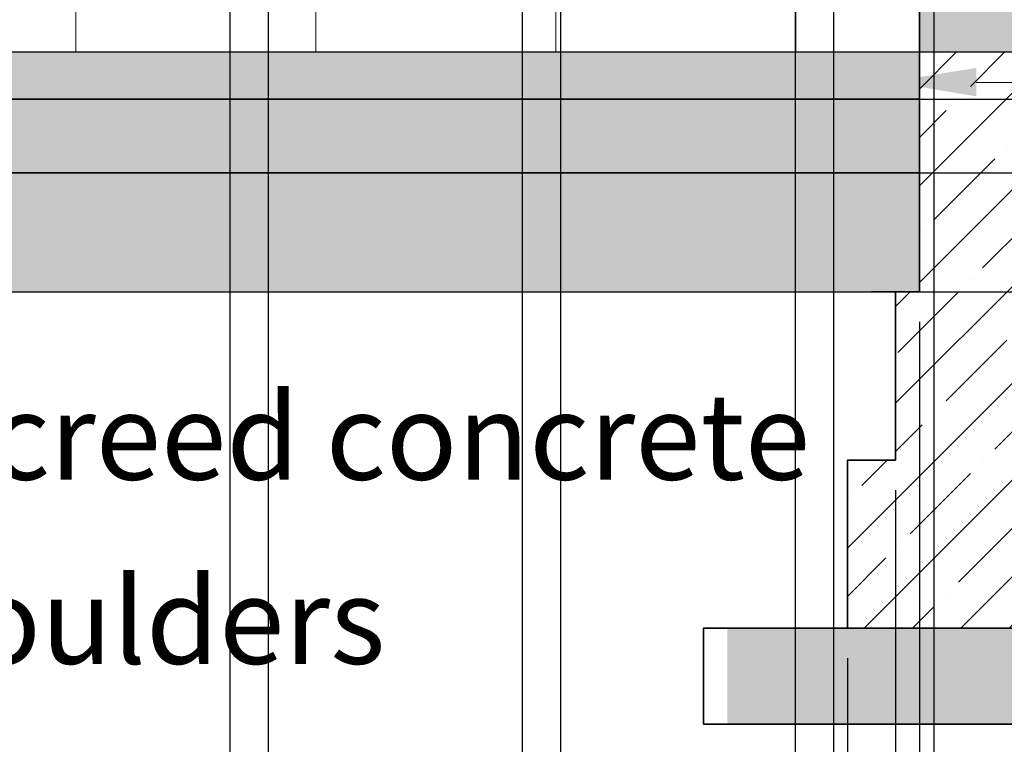
# Model space of a CAD drawing. Units: metres. Extents: x 22.1 to 34.4, y 4.4 to 12.4.
# Tile 4 of 8: x 29.6 to 31.7, y 7 to 8.5. Entities that reach past the tile are written whole.
import ezdxf
from ezdxf import colors
from ezdxf.entities.mleader import LeaderData, LeaderLine
from ezdxf.math import Vec2, Vec3

# ---------------------------------------------------------------- set-up
doc = ezdxf.new("R2010")
doc.units = ezdxf.units.M
doc.header["$MEASUREMENT"] = 0
for name, color, linetype, lineweight in [('A-ANNO-DIMS', 2, 'Continuous', 18), ('A-ANNO-TEXT', 7, 'Continuous', 18), ('A-FLOR', 3, 'Continuous', 25), ('A-FLOR-PATT', 252, 'Continuous', 13), ('S-FNDN', 1, 'Continuous', 35), ('S-FNDN-PATT', 8, 'Continuous', 13), ('S-SLAB-PATT', 8, 'Continuous', 13)]:
    doc.layers.add(name, color=color, linetype=linetype, lineweight=lineweight)
doc.styles.get("Standard").update_dxf_attribs({"font": 'arial.ttf'})
doc.dimstyles.get("Standard").update_dxf_attribs({"dimtxt": 0.18, "dimasz": 0.18, "dimexe": 0.18, "dimexo": 0.0625, "dimgap": 0.09, "dimtad": 0, "dimtih": 1, "dimtoh": 1, "dimzin": 0, "dimdsep": 46, "dimtxsty": 'Standard', "dimcen": 0.09, "dimadec": 0, "dimazin": 0, "dimtfac": 1, "dimtofl": 0, "dimtmove": 0, "dimatfit": 3, "dimfxl": 1, "dimtolj": 1, "dimtzin": 0, "dimarcsym": 0})

# ---------------------------------------------------------------- blocks, each defined once
blk = doc.blocks.new('*D7')
at = {"layer": 'A-ANNO-DIMS', "color": 0, "lineweight": -2, "transparency": 16777216}
for p, q in [((31.0581, 6.9474), (31.0581, 5.2806)), ((32.2581, 6.9474), (32.2581, 5.2806)), ((31.0581, 5.4606), (30.8781, 5.4606)), ((32.0781, 5.4606), (31.2381, 5.4606))]:
    blk.add_line(p, q, dxfattribs=at)
at = {"layer": 'A-ANNO-DIMS', "color": 0, "transparency": 16777216}
for points in [[(31.2381, 5.4906), (31.2381, 5.4306), (31.0581, 5.4606)], [(32.0781, 5.4906), (32.0781, 5.4306), (32.2581, 5.4606)]]:
    blk.add_solid(points, dxfattribs=at)
at = {"layer": 'Defpoints', "color": 0, "transparency": 16777216}
for p in [(31.0581, 7.0099), (32.2581, 7.0099), (32.2581, 5.4606)]:
    blk.add_point(p, dxfattribs=at)
at = {"layer": 'A-ANNO-DIMS', "color": 0, "transparency": 16777216, "insert": (30.5631, 5.4606), "char_height": 0.18, "attachment_point": 5}
blk.add_mtext('\\A1;1.20', dxfattribs=at)
blk = doc.blocks.new('*D8')
at = {"layer": 'A-ANNO-DIMS', "color": 0, "lineweight": -2, "transparency": 16777216}
for p, q in [((31.3581, 7.1474), (31.3581, 5.6208)), ((31.9581, 7.1474), (31.9581, 5.6208)), ((31.3581, 5.8008), (30.8904, 5.8008)), ((31.7781, 5.8008), (31.5381, 5.8008))]:
    blk.add_line(p, q, dxfattribs=at)
at = {"layer": 'A-ANNO-DIMS', "color": 0, "transparency": 16777216}
for points in [[(31.5381, 5.8308), (31.5381, 5.7708), (31.3581, 5.8008)], [(31.7781, 5.8308), (31.7781, 5.7708), (31.9581, 5.8008)]]:
    blk.add_solid(points, dxfattribs=at)
at = {"layer": 'Defpoints', "color": 0, "transparency": 16777216}
for p in [(31.3581, 7.2099), (31.9581, 7.2099), (31.9581, 5.8008)]:
    blk.add_point(p, dxfattribs=at)
at = {"layer": 'A-ANNO-DIMS', "color": 0, "transparency": 16777216, "insert": (30.5669, 5.8008), "char_height": 0.18, "attachment_point": 5}
blk.add_mtext('\\A1;0.60', dxfattribs=at)
blk = doc.blocks.new('*D9')
at = {"layer": 'A-ANNO-DIMS', "color": 0, "lineweight": -2, "transparency": 16777216}
for p, q in [((31.4581, 7.4974), (31.4581, 5.952)), ((31.8581, 7.4974), (31.8581, 5.952)), ((31.2781, 6.132), (30.8756, 6.132)), ((32.0381, 6.132), (32.2181, 6.132))]:
    blk.add_line(p, q, dxfattribs=at)
at = {"layer": 'A-ANNO-DIMS', "color": 0, "transparency": 16777216}
for points in [[(31.2781, 6.162), (31.2781, 6.102), (31.4581, 6.132)], [(32.0381, 6.162), (32.0381, 6.102), (31.8581, 6.132)]]:
    blk.add_solid(points, dxfattribs=at)
at = {"layer": 'Defpoints', "color": 0, "transparency": 16777216}
for p in [(31.4581, 7.5599), (31.8581, 7.5599), (31.8581, 6.132)]:
    blk.add_point(p, dxfattribs=at)
at = {"layer": 'A-ANNO-DIMS', "color": 0, "transparency": 16777216, "insert": (30.5521, 6.132), "char_height": 0.18, "attachment_point": 5}
blk.add_mtext('\\A1;0.40', dxfattribs=at)
blk = doc.blocks.new('*D10')
at = {"layer": 'A-ANNO-DIMS', "color": 0, "lineweight": -2, "transparency": 16777216}
for p, q in [((31.5081, 7.8474), (31.5081, 6.2035)), ((31.8081, 7.8474), (31.8081, 6.2035)), ((31.3281, 6.3835), (30.8854, 6.3835)), ((31.9881, 6.3835), (32.1681, 6.3835))]:
    blk.add_line(p, q, dxfattribs=at)
at = {"layer": 'A-ANNO-DIMS', "color": 0, "transparency": 16777216}
for points in [[(31.3281, 6.4135), (31.3281, 6.3535), (31.5081, 6.3835)], [(31.9881, 6.4135), (31.9881, 6.3535), (31.8081, 6.3835)]]:
    blk.add_solid(points, dxfattribs=at)
at = {"layer": 'Defpoints', "color": 0, "transparency": 16777216}
for p in [(31.5081, 7.9099), (31.8081, 7.9099), (31.8081, 6.3835)]:
    blk.add_point(p, dxfattribs=at)
at = {"layer": 'A-ANNO-DIMS', "color": 0, "transparency": 16777216, "insert": (30.562, 6.3835), "char_height": 0.18, "attachment_point": 5}
blk.add_mtext('\\A1;0.30', dxfattribs=at)
blk = doc.blocks.new('*D23')
at = {"layer": 'A-ANNO-DIMS', "color": 0, "lineweight": -2, "transparency": 16777216}
for p, q in [((28.0901, 11.4474), (28.0901, 6.2449)), ((31.5381, 11.4474), (31.5381, 6.2449)), ((28.2701, 6.4249), (29.4202, 6.4249)), ((31.3581, 6.4249), (30.2079, 6.4249))]:
    blk.add_line(p, q, dxfattribs=at)
at = {"layer": 'A-ANNO-DIMS', "color": 0, "transparency": 16777216}
for points in [[(28.2701, 6.4549), (28.2701, 6.3949), (28.0901, 6.4249)], [(31.3581, 6.4549), (31.3581, 6.3949), (31.5381, 6.4249)]]:
    blk.add_solid(points, dxfattribs=at)
at = {"layer": 'Defpoints', "color": 0, "transparency": 16777216}
for p in [(28.0901, 11.5099), (31.5381, 11.5099), (31.5381, 6.4249)]:
    blk.add_point(p, dxfattribs=at)
at = {"layer": 'A-ANNO-DIMS', "color": 0, "transparency": 16777216, "insert": (29.8141, 6.4249), "char_height": 0.18, "attachment_point": 5}
blk.add_mtext('\\A1;3.448', dxfattribs=at)
blk = doc.blocks.new('*D27')
at = {"layer": 'A-ANNO-DIMS', "color": 0, "lineweight": -2, "transparency": 16777216}
for p, q in [((31.5381, 11.4474), (31.5381, 6.2449)), ((31.7781, 11.4474), (31.7781, 6.2449)), ((31.3581, 6.4249), (31.1781, 6.4249)), ((31.9581, 6.4249), (32.1381, 6.4249))]:
    blk.add_line(p, q, dxfattribs=at)
at = {"layer": 'A-ANNO-DIMS', "color": 0, "transparency": 16777216}
for points in [[(31.3581, 6.4549), (31.3581, 6.3949), (31.5381, 6.4249)], [(31.9581, 6.4549), (31.9581, 6.3949), (31.7781, 6.4249)]]:
    blk.add_solid(points, dxfattribs=at)
at = {"layer": 'Defpoints', "color": 0, "transparency": 16777216}
for p in [(31.5381, 11.5099), (31.7781, 11.5099), (31.7781, 6.4249)]:
    blk.add_point(p, dxfattribs=at)
at = {"layer": 'A-ANNO-DIMS', "color": 0, "transparency": 16777216, "insert": (32.4615, 6.4249), "char_height": 0.18, "attachment_point": 5}
blk.add_mtext('\\A1;0.24', dxfattribs=at)
blk = doc.blocks.new('*D28')
at = {"layer": 'A-ANNO-DIMS', "color": 0, "lineweight": -2, "transparency": 16777216}
for p, q in [((31.7781, 11.4474), (31.7781, 6.2449)), ((31.9781, 11.4474), (31.9781, 6.2449)), ((31.5981, 6.4249), (31.4181, 6.4249)), ((32.1581, 6.4249), (32.3381, 6.4249))]:
    blk.add_line(p, q, dxfattribs=at)
at = {"layer": 'A-ANNO-DIMS', "color": 0, "transparency": 16777216}
for points in [[(31.5981, 6.4549), (31.5981, 6.3949), (31.7781, 6.4249)], [(32.1581, 6.4549), (32.1581, 6.3949), (31.9781, 6.4249)]]:
    blk.add_solid(points, dxfattribs=at)
at = {"layer": 'Defpoints', "color": 0, "transparency": 16777216}
for p in [(31.7781, 11.5099), (31.9781, 11.5099), (31.9781, 6.4249)]:
    blk.add_point(p, dxfattribs=at)
at = {"layer": 'A-ANNO-DIMS', "color": 0, "transparency": 16777216, "insert": (32.6615, 6.4249), "char_height": 0.18, "attachment_point": 5}
blk.add_mtext('\\A1;0.20', dxfattribs=at)
blk = doc.blocks.new('*D33')
at = {"layer": 'A-ANNO-DIMS', "color": 0, "lineweight": -2, "transparency": 16777216}
for p, q in [((31.5381, 11.4474), (31.5381, 6.2449)), ((31.3293, 10.5774), (31.3293, 6.2449)), ((31.1493, 6.4249), (30.9693, 6.4249)), ((31.7181, 6.4249), (31.8981, 6.4249))]:
    blk.add_line(p, q, dxfattribs=at)
at = {"layer": 'A-ANNO-DIMS', "color": 0, "transparency": 16777216}
for points in [[(31.1493, 6.4549), (31.1493, 6.3949), (31.3293, 6.4249)], [(31.7181, 6.4549), (31.7181, 6.3949), (31.5381, 6.4249)]]:
    blk.add_solid(points, dxfattribs=at)
at = {"layer": 'Defpoints', "color": 0, "transparency": 16777216}
for p in [(31.5381, 11.5099), (31.3293, 10.6399), (31.5381, 6.4249)]:
    blk.add_point(p, dxfattribs=at)
at = {"layer": 'A-ANNO-DIMS', "color": 0, "transparency": 16777216, "insert": (32.2045, 6.4249), "char_height": 0.18, "attachment_point": 5}
blk.add_mtext('\\A1;0.21', dxfattribs=at)
blk = doc.blocks.new('*D34')
at = {"layer": 'A-ANNO-DIMS', "color": 0, "lineweight": -2, "transparency": 16777216}
for p, q in [((28.8933, 9.3614), (28.8933, 6.2449)), ((31.3293, 9.3614), (31.3293, 6.2449)), ((29.0733, 6.4249), (29.7162, 6.4249)), ((31.1493, 6.4249), (30.5065, 6.4249))]:
    blk.add_line(p, q, dxfattribs=at)
at = {"layer": 'A-ANNO-DIMS', "color": 0, "transparency": 16777216}
for points in [[(29.0733, 6.4549), (29.0733, 6.3949), (28.8933, 6.4249)], [(31.1493, 6.4549), (31.1493, 6.3949), (31.3293, 6.4249)]]:
    blk.add_solid(points, dxfattribs=at)
at = {"layer": 'Defpoints', "color": 0, "transparency": 16777216}
for p in [(28.8933, 9.4239), (31.3293, 9.4239), (31.3293, 6.4249)]:
    blk.add_point(p, dxfattribs=at)
at = {"layer": 'A-ANNO-DIMS', "color": 0, "transparency": 16777216, "insert": (30.1113, 6.4249), "char_height": 0.18, "attachment_point": 5}
blk.add_mtext('\\A1;2.436', dxfattribs=at)
blk = doc.blocks.new('*D35')
at = {"layer": 'A-ANNO-DIMS', "color": 0, "lineweight": -2, "transparency": 16777216}
for p, q in [((28.9733, 9.4414), (28.9733, 6.2449)), ((28.8933, 9.3614), (28.8933, 6.2449)), ((28.7133, 6.4249), (28.5333, 6.4249)), ((29.1533, 6.4249), (29.3333, 6.4249))]:
    blk.add_line(p, q, dxfattribs=at)
at = {"layer": 'A-ANNO-DIMS', "color": 0, "transparency": 16777216}
for points in [[(28.7133, 6.4549), (28.7133, 6.3949), (28.8933, 6.4249)], [(29.1533, 6.4549), (29.1533, 6.3949), (28.9733, 6.4249)]]:
    blk.add_solid(points, dxfattribs=at)
at = {"layer": 'Defpoints', "color": 0, "transparency": 16777216}
for p in [(28.9733, 9.5039), (28.8933, 9.4239), (28.9733, 6.4249)]:
    blk.add_point(p, dxfattribs=at)
at = {"layer": 'A-ANNO-DIMS', "color": 0, "transparency": 16777216, "insert": (29.6573, 6.4249), "char_height": 0.18, "attachment_point": 5}
blk.add_mtext('\\A1;0.08', dxfattribs=at)
blk = doc.blocks.new('*D36')
at = {"layer": 'A-ANNO-DIMS', "color": 0, "lineweight": -2, "transparency": 16777216}
for p, q in [((29.4623, 9.4414), (29.4623, 6.2449)), ((29.5423, 9.4414), (29.5423, 6.2449)), ((29.2823, 6.4249), (29.1023, 6.4249)), ((29.7223, 6.4249), (29.9023, 6.4249))]:
    blk.add_line(p, q, dxfattribs=at)
at = {"layer": 'A-ANNO-DIMS', "color": 0, "transparency": 16777216}
for points in [[(29.2823, 6.4549), (29.2823, 6.3949), (29.4623, 6.4249)], [(29.7223, 6.4549), (29.7223, 6.3949), (29.5423, 6.4249)]]:
    blk.add_solid(points, dxfattribs=at)
at = {"layer": 'Defpoints', "color": 0, "transparency": 16777216}
for p in [(29.4623, 9.5039), (29.5423, 9.5039), (29.5423, 6.4249)]:
    blk.add_point(p, dxfattribs=at)
at = {"layer": 'A-ANNO-DIMS', "color": 0, "transparency": 16777216, "insert": (30.2263, 6.4249), "char_height": 0.18, "attachment_point": 5}
blk.add_mtext('\\A1;0.08', dxfattribs=at)
blk = doc.blocks.new('*D37')
at = {"layer": 'A-ANNO-DIMS', "color": 0, "lineweight": -2, "transparency": 16777216}
for p, q in [((30.0713, 9.4414), (30.0713, 6.2449)), ((30.1513, 9.4414), (30.1513, 6.2449)), ((29.8913, 6.4249), (29.7113, 6.4249)), ((30.3313, 6.4249), (30.5113, 6.4249))]:
    blk.add_line(p, q, dxfattribs=at)
at = {"layer": 'A-ANNO-DIMS', "color": 0, "transparency": 16777216}
for points in [[(29.8913, 6.4549), (29.8913, 6.3949), (30.0713, 6.4249)], [(30.3313, 6.4549), (30.3313, 6.3949), (30.1513, 6.4249)]]:
    blk.add_solid(points, dxfattribs=at)
at = {"layer": 'Defpoints', "color": 0, "transparency": 16777216}
for p in [(30.0713, 9.5039), (30.1513, 9.5039), (30.1513, 6.4249)]:
    blk.add_point(p, dxfattribs=at)
at = {"layer": 'A-ANNO-DIMS', "color": 0, "transparency": 16777216, "insert": (30.8353, 6.4249), "char_height": 0.18, "attachment_point": 5}
blk.add_mtext('\\A1;0.08', dxfattribs=at)
blk = doc.blocks.new('*D38')
at = {"layer": 'A-ANNO-DIMS', "color": 0, "lineweight": -2, "transparency": 16777216}
for p, q in [((30.6803, 9.4414), (30.6803, 6.2449)), ((30.7603, 9.4414), (30.7603, 6.2449)), ((30.5003, 6.4249), (30.3203, 6.4249)), ((30.9403, 6.4249), (31.1203, 6.4249))]:
    blk.add_line(p, q, dxfattribs=at)
at = {"layer": 'A-ANNO-DIMS', "color": 0, "transparency": 16777216}
for points in [[(30.5003, 6.4549), (30.5003, 6.3949), (30.6803, 6.4249)], [(30.9403, 6.4549), (30.9403, 6.3949), (30.7603, 6.4249)]]:
    blk.add_solid(points, dxfattribs=at)
at = {"layer": 'Defpoints', "color": 0, "transparency": 16777216}
for p in [(30.6803, 9.5039), (30.7603, 9.5039), (30.7603, 6.4249)]:
    blk.add_point(p, dxfattribs=at)
at = {"layer": 'A-ANNO-DIMS', "color": 0, "transparency": 16777216, "insert": (31.4443, 6.4249), "char_height": 0.18, "attachment_point": 5}
blk.add_mtext('\\A1;0.08', dxfattribs=at)
blk = doc.blocks.new('*D39')
at = {"layer": 'A-ANNO-DIMS', "color": 0, "lineweight": -2, "transparency": 16777216}
for p, q in [((31.2493, 9.4414), (31.2493, 6.2449)), ((31.3293, 9.3614), (31.3293, 6.2449)), ((31.0693, 6.4249), (30.8893, 6.4249)), ((31.5093, 6.4249), (31.6893, 6.4249))]:
    blk.add_line(p, q, dxfattribs=at)
at = {"layer": 'A-ANNO-DIMS', "color": 0, "transparency": 16777216}
for points in [[(31.0693, 6.4549), (31.0693, 6.3949), (31.2493, 6.4249)], [(31.5093, 6.4549), (31.5093, 6.3949), (31.3293, 6.4249)]]:
    blk.add_solid(points, dxfattribs=at)
at = {"layer": 'Defpoints', "color": 0, "transparency": 16777216}
for p in [(31.2493, 9.5039), (31.3293, 9.4239), (31.3293, 6.4249)]:
    blk.add_point(p, dxfattribs=at)
at = {"layer": 'A-ANNO-DIMS', "color": 0, "transparency": 16777216, "insert": (32.0133, 6.4249), "char_height": 0.18, "attachment_point": 5}
blk.add_mtext('\\A1;0.08', dxfattribs=at)
blk = doc.blocks.new('*D44')
at = {"layer": 'A-ANNO-DIMS', "color": 0, "lineweight": -2, "transparency": 16777216}
for p, q in [((33.6737, 8.6899), (33.6737, 8.8699)), ((24.8474, 8.5099), (33.8537, 8.5099)), ((24.5474, 8.4099), (33.8537, 8.4099)), ((33.6737, 8.2299), (33.6737, 8.0499)), ((33.6737, 8.0499), (33.4937, 8.0499))]:
    blk.add_line(p, q, dxfattribs=at)
at = {"layer": 'A-ANNO-DIMS', "color": 0, "transparency": 16777216}
for points in [[(33.6437, 8.6899), (33.7037, 8.6899), (33.6737, 8.5099)], [(33.6437, 8.2299), (33.7037, 8.2299), (33.6737, 8.4099)]]:
    blk.add_solid(points, dxfattribs=at)
at = {"layer": 'Defpoints', "color": 0, "transparency": 16777216}
for p in [(24.7849, 8.5099), (24.4849, 8.4099), (33.6737, 8.4099)]:
    blk.add_point(p, dxfattribs=at)
at = {"layer": 'A-ANNO-DIMS', "color": 0, "transparency": 16777216, "insert": (33.1702, 8.0499), "char_height": 0.18, "attachment_point": 5}
blk.add_mtext('\\A1;0.10', dxfattribs=at)
blk = doc.blocks.new('*D45')
at = {"layer": 'A-ANNO-DIMS', "color": 0, "lineweight": -2, "transparency": 16777216}
for p, q in [((33.6737, 8.5899), (33.6737, 8.7699)), ((24.5474, 8.4099), (33.8537, 8.4099)), ((24.8474, 8.3119), (33.8537, 8.3119)), ((33.6737, 8.1319), (33.6737, 7.9519)), ((33.6737, 7.9519), (33.4937, 7.9519))]:
    blk.add_line(p, q, dxfattribs=at)
at = {"layer": 'A-ANNO-DIMS', "color": 0, "transparency": 16777216}
for points in [[(33.6437, 8.5899), (33.7037, 8.5899), (33.6737, 8.4099)], [(33.6437, 8.1319), (33.7037, 8.1319), (33.6737, 8.3119)]]:
    blk.add_solid(points, dxfattribs=at)
at = {"layer": 'Defpoints', "color": 0, "transparency": 16777216}
for p in [(24.4849, 8.4099), (24.7849, 8.3119), (33.6737, 8.3119)]:
    blk.add_point(p, dxfattribs=at)
at = {"layer": 'A-ANNO-DIMS', "color": 0, "transparency": 16777216, "insert": (33.0998, 7.9519), "char_height": 0.18, "attachment_point": 5}
blk.add_mtext('\\A1;0.098', dxfattribs=at)
blk = doc.blocks.new('*D46')
at = {"layer": 'A-ANNO-DIMS', "color": 0, "lineweight": -2, "transparency": 16777216}
for p, q in [((33.6737, 8.4919), (33.6737, 8.6719)), ((24.8474, 8.3119), (33.8537, 8.3119)), ((24.8474, 8.1578), (33.8537, 8.1578)), ((33.6737, 7.9778), (33.6737, 7.7978)), ((33.6737, 7.7978), (33.4937, 7.7978))]:
    blk.add_line(p, q, dxfattribs=at)
at = {"layer": 'A-ANNO-DIMS', "color": 0, "transparency": 16777216}
for points in [[(33.6437, 8.4919), (33.7037, 8.4919), (33.6737, 8.3119)], [(33.6437, 7.9778), (33.7037, 7.9778), (33.6737, 8.1578)]]:
    blk.add_solid(points, dxfattribs=at)
at = {"layer": 'Defpoints', "color": 0, "transparency": 16777216}
for p in [(24.7849, 8.3119), (24.7849, 8.1578), (33.6737, 8.1578)]:
    blk.add_point(p, dxfattribs=at)
at = {"layer": 'A-ANNO-DIMS', "color": 0, "transparency": 16777216, "insert": (33.1692, 7.7978), "char_height": 0.18, "attachment_point": 5}
blk.add_mtext('\\A1;0.15', dxfattribs=at)
blk = doc.blocks.new('*D47')
at = {"layer": 'A-ANNO-DIMS', "color": 0, "lineweight": -2, "transparency": 16777216}
for p, q in [((33.6737, 8.3378), (33.6737, 8.5178)), ((24.8474, 8.1578), (33.8537, 8.1578)), ((24.8474, 7.9099), (33.8537, 7.9099)), ((33.6737, 7.7299), (33.6737, 7.5499)), ((33.6737, 7.5499), (33.4937, 7.5499))]:
    blk.add_line(p, q, dxfattribs=at)
at = {"layer": 'A-ANNO-DIMS', "color": 0, "transparency": 16777216}
for points in [[(33.6437, 8.3378), (33.7037, 8.3378), (33.6737, 8.1578)], [(33.6437, 7.7299), (33.7037, 7.7299), (33.6737, 7.9099)]]:
    blk.add_solid(points, dxfattribs=at)
at = {"layer": 'Defpoints', "color": 0, "transparency": 16777216}
for p in [(24.7849, 8.1578), (24.7849, 7.9099), (33.6737, 7.9099)]:
    blk.add_point(p, dxfattribs=at)
at = {"layer": 'A-ANNO-DIMS', "color": 0, "transparency": 16777216, "insert": (33.1692, 7.5499), "char_height": 0.18, "attachment_point": 5}
blk.add_mtext('\\A1;0.25', dxfattribs=at)

msp = doc.modelspace()

# ---------------------------------------------------------------- hatches: boundary and pattern name
at = {"layer": 'A-FLOR-PATT'}
h = msp.add_hatch(dxfattribs=at)
h.set_pattern_fill('BRICK', color=256)
h.paths.add_polyline_path([(31.5081, 8.5099), (28.1201, 8.5099), (28.1201, 8.4099), (31.5081, 8.4099)])
h.paths.add_polyline_path([(27.8201, 8.5099), (27.0468, 8.5099), (26.6456, 8.5099), (26.6456, 8.4099), (27.8201, 8.4099)])
h.paths.add_polyline_path([(26.3456, 8.5099), (25.6173, 8.5099), (24.7849, 8.5099), (24.7849, 8.4099), (26.3456, 8.4099)])
h = msp.add_hatch(dxfattribs=at)
h.set_pattern_fill('AR-SAND', color=256, scale=0.57)
h.paths.add_polyline_path([(26.3456, 8.4099), (24.7849, 8.4099), (24.7849, 8.3119), (26.3456, 8.3119)])
h.paths.add_polyline_path([(27.8201, 8.4099), (26.6456, 8.4099), (26.6456, 8.3119), (27.8201, 8.3119)])
h.paths.add_polyline_path([(31.5081, 8.4099), (28.1201, 8.4099), (28.1201, 8.3119), (31.5081, 8.3119)])
h = msp.add_hatch(dxfattribs=at)
h.set_pattern_fill('AR-SAND', color=256, scale=0.57)
h.paths.add_polyline_path([(31.5081, 8.4099), (28.1201, 8.4099), (28.1201, 8.3119), (31.5081, 8.3119)])
h.paths.add_polyline_path([(27.8201, 8.4099), (26.6456, 8.4099), (26.6456, 8.3119), (27.8201, 8.3119)])
h.paths.add_polyline_path([(26.3456, 8.4099), (24.7849, 8.4099), (24.7849, 8.3119), (26.3456, 8.3119)])
h = msp.add_hatch(dxfattribs=at)
h.set_pattern_fill('AR-SAND', color=256, scale=0.04)
h.paths.add_polyline_path([(26.3456, 8.4099), (24.7849, 8.4099), (24.7849, 8.3119), (26.3456, 8.3119)])
h.paths.add_polyline_path([(27.8201, 8.4099), (26.6456, 8.4099), (26.6456, 8.3119), (27.8201, 8.3119)])
h.paths.add_polyline_path([(31.5081, 8.4099), (28.1201, 8.4099), (28.1201, 8.3119), (31.5081, 8.3119)])
h = msp.add_hatch(dxfattribs=at)
h.set_pattern_fill('GRAVEL', color=256, scale=0.18)
h.set_pattern_definition([(228.012788, (0.1296, 0.18), (-1.44, -1.62), [0.0242165, -2.39743585]), (184.96974, (0.1134, 0.162), (2.16, 0.18), [0.0415562, -4.1140665]), (132.510447, (0.072, 0.1584), (1.8, -1.98), [0.0293018, -2.9008859]), (267.27369, (0.0018, 0.1134), (0.18, 3.6), [0.0378428, -3.74644045]), (292.833654, (0, 0.0756), (-0.9, 2.16), [0.0371079, -3.6736872]), (357.27369, (0.0144, 0.0414), (-3.6, 0.18), [0.0378428, -3.74644045]), (37.69424, (0.0522, 0.0396), (-2.34, -1.8), [0.0500452, -4.9544727]), (72.255328, (0.0918, 0.0702), (1.26, 3.96), [0.0472478, -4.6775379]), (121.429566, (0.1062, 0.1152), (-1.44, 2.34), [0.037971, -3.7591332]), (175.23636, (0.0864, 0.1476), (1.98, -0.18), [0.0433498, -2.1241373]), (222.397438, (0.0432, 0.1512), (-2.16, -1.98), [0.0560606, -5.5500075]), (138.814075, (0.18, 0.1116), (-1.26, 1.08), [0.0191342, -1.8942921]), (171.469234, (0.1656, 0.1242), (2.34, -0.36), [0.0364027, -3.60387205]), (225, (0.1296, 0.1296), (0, -0.18), [0.0254558, -0.2291027]), (203.19859, (0.117, 0.1512), (0.9, 0.36), [0.0137084, -1.3571307]), (291.80141, (0.1044, 0.1458), (-0.18, 0.54), [0.0193865, -0.9499431]), (30.96376, (0.1116, 0.1278), (0.54, 0.36), [0.0314872, -1.0180841]), (161.56505, (0.1386, 0.144), (0.36, -0.18), [0.0227684, -0.5464416]), (16.38954, (0, 0.1458), (1.8, 0.54), [0.031896, -3.1577121]), (70.346176, (0.0306, 0.1548), (-0.72, -1.98), [0.026759, -2.6491334]), (293.19859, (0.1386, 0.18), (-0.36, 0.9), [0.0274167, -1.3434225]), (343.61046, (0.1494, 0.1548), (-1.8, 0.54), [0.031896, -3.1577121]), (339.443955, (0, 0.0342), (-0.9, 0.36), [0.0307584, -1.5071623]), (294.77514, (0.0288, 0.0234), (-0.9, 1.98), [0.025772, -2.55143575]), (66.80141, (0.1404, 0), (0.36, 0.9), [0.0274167, -1.3434225]), (17.354025, (0.1512, 0.0252), (-2.34, -0.72), [0.0301736, -2.98717625]), (69.443955, (0.0522, 0), (-0.36, -0.9), [0.0153792, -1.5225415]), (101.30993, (0.1296, 0), (-0.18, 0.72), [0.0091782, -0.9086453]), (165.96376, (0.1278, 0.009), (0.54, -0.18), [0.0371079, -0.7050511]), (186.009006, (0.0918, 0.018), (1.8, 0.18), [0.034389, -3.4045062]), (303.69007, (0.1116, 0.1116), (-0.18, 0.36), [0.02596, -0.6230393]), (353.157227, (0.126, 0.09), (3.06, -0.36), [0.0453229, -4.4869613]), (60.945396, (0.171, 0.0846), (-0.72, -1.26), [0.0185321, -1.8346813]), (90, (0.18, 0.1008), (-0.18, 0.18), [0.0108, -0.1692]), (120.256437, (0.0882, 0.0234), (0.72, -1.26), [0.0250063, -2.4756336]), (48.012788, (0.0756, 0.045), (1.44, 1.62), [0.048433, -2.3732194]), (0, (0.108, 0.081), (0.18, 0.18), [0.0468, -0.1332]), (325.304846, (0.1548, 0.081), (1.8, -1.26), [0.0284605, -2.8175894]), (254.0546, (0.1782, 0.0648), (-0.18, -0.72), [0.0262084, -1.2842114]), (207.645975, (0.171, 0.0396), (-3.42, -1.8), [0.0426717, -4.22450535]), (175.42608, (0.1332, 0.0198), (-2.34, 0.18), [0.0451438, -4.4692332])])
h.paths.add_polyline_path([(26.3456, 8.1578), (24.7849, 8.1578), (24.7849, 7.9099), (24.8849, 7.9099), (26.3456, 7.9099)])
h.paths.add_polyline_path([(27.8201, 8.1578), (26.6456, 8.1578), (26.6456, 7.9099), (26.7456, 7.9099), (27.8201, 7.9099)])
h.paths.add_polyline_path([(31.5081, 8.1578), (28.1201, 8.1578), (28.1201, 7.9099), (31.4081, 7.9099), (31.5081, 7.9099)])
at = {"layer": 'S-FNDN-PATT'}
h = msp.add_hatch(dxfattribs=at)
h.set_pattern_fill('ANSI35', color=256, scale=0.57)
h.paths.add_polyline_path([(24.3849, 7.5599), (24.2849, 7.5599), (24.2849, 7.2099), (24.9849, 7.2099), (24.9849, 7.5599), (24.8849, 7.5599), (24.8849, 7.9099), (24.7849, 7.9099), (24.7849, 8.4099), (24.4849, 8.4099), (24.4849, 7.9099), (24.3849, 7.9099)])
h.paths.add_polyline_path([(27.7201, 7.5599), (27.6201, 7.5599), (27.6201, 7.2099), (28.3201, 7.2099), (28.3201, 7.5599), (28.2201, 7.5599), (28.2201, 7.9099), (28.1201, 7.9099), (28.1201, 8.4099), (27.8201, 8.4099), (27.8201, 7.9099), (27.7201, 7.9099)])
h.paths.add_polyline_path([(26.7456, 7.9099), (26.6456, 7.9099), (26.6456, 8.4099), (26.3456, 8.4099), (26.3456, 7.9099), (26.2456, 7.9099), (26.2456, 7.5599), (26.4616, 7.5599), (26.4616, 7.6127), (26.4825, 7.5003), (26.4825, 7.5599), (26.7456, 7.5599)])
h.paths.add_polyline_path([(31.8581, 7.5599), (31.8581, 7.9099), (31.8081, 7.9099), (31.8081, 8.4099), (31.5081, 8.4099), (31.5081, 7.9099), (31.4581, 7.9099), (31.4581, 7.5599), (31.3581, 7.5599), (31.3581, 7.2099), (31.9581, 7.2099), (31.9581, 7.5599)])
at = {"layer": 'S-SLAB-PATT'}
h = msp.add_hatch(dxfattribs=at)
h.set_pattern_fill('AR-CONC', color=256, scale=0.04)
h.set_pattern_definition([(50, (0, 0), (0.286904, -0.0251009), [0.03, -0.33]), (355, (0, 0), (-0.0555005, 0.3008769), [0.024, -0.264]), (100.4514, (0.0239, -0.0021), (0.2314035, 0.275776), [0.025496, -0.2804568]), (46.1842, (0, 0.08), (0.4268965, -0.0662077), [0.045, -0.495]), (96.6356, (0.03557, 0.0745), (0.373865, 0.3896474), [0.038244, -0.4206855]), (351.1842, (0, 0.08), (0.373865, 0.3896474), [0.036, -0.396]), (21, (0.04, 0.06), (0.2387628, -0.1610476), [0.03, -0.33]), (326, (0.04, 0.06), (0.0973261, 0.29006), [0.024, -0.264]), (71.4514, (0.0599, 0.04658), (0.336089, 0.1290125), [0.025496, -0.2804568]), (37.5, (0, 0), (0.00486394, 0.13315754), [0, -0.2608, 0, -0.268, 0, -0.265]), (7.5, (0, 0), (0.1052278, 0.1577647), [0, -0.1528, 0, -0.2548, 0, -0.101]), (327.5, (-0.0892, 0), (0.21352897, -0.00902195), [0, -0.1, 0, -0.312, 0, -0.414]), (317.5, (-0.1292, 0), (0.2332745, 0.040042), [0, -0.13, 0, -0.2072, 0, -0.294])])
h.paths.add_polyline_path([(31.9781, 11.6599), (24.3149, 11.6599), (24.3149, 11.5099), (24.5149, 11.5099), (31.7781, 11.5099), (31.9781, 11.5099)])
h.paths.add_polyline_path([(25.1849, 7.2099), (24.9849, 7.2099), (24.0849, 7.2099), (24.0849, 7.0099), (25.1849, 7.0099)])
h.paths.add_polyline_path([(32.2081, 7.2099), (32.0081, 7.2099), (31.1081, 7.2099), (31.1081, 7.0099), (32.2081, 7.0099)])
h.paths.add_polyline_path([(28.5201, 7.2099), (28.3201, 7.2099), (27.4201, 7.2099), (27.4201, 7.0099), (28.5201, 7.0099)])
h.paths.add_polyline_path([(24.7849, 8.5099), (24.6349, 8.5099), (24.5149, 8.5099), (24.4849, 8.5099), (24.4849, 8.4099), (24.7849, 8.4099)])
h.paths.add_polyline_path([(26.6456, 8.5099), (26.3456, 8.5099), (26.3456, 8.4099), (26.6456, 8.4099)])
h.paths.add_polyline_path([(28.1201, 8.5099), (28.0901, 8.5099), (27.8201, 8.5099), (27.8201, 8.4099), (28.1201, 8.4099)])
h.paths.add_polyline_path([(31.8081, 8.5099), (31.6581, 8.5099), (31.5381, 8.5099), (31.5081, 8.5099), (31.5081, 8.4099), (31.8081, 8.4099)])
h.paths.add_polyline_path([(26.3456, 8.3119), (24.7849, 8.3119), (24.7849, 8.1578), (26.3456, 8.1578)])
h.paths.add_polyline_path([(27.8201, 8.3119), (26.6456, 8.3119), (26.6456, 8.1578), (27.8201, 8.1578)])
h.paths.add_polyline_path([(31.5081, 8.3119), (28.1201, 8.3119), (28.1201, 8.1578), (31.5081, 8.1578)])

# ---------------------------------------------------------------- linework, layer by layer
at = {"layer": 'A-FLOR'}
for p, q in [((28.1201, 8.4099), (31.8081, 8.4099)), ((31.5081, 8.3119), (28.1201, 8.3119)), ((31.5081, 8.1578), (28.1201, 8.1578)), ((28.1201, 7.9099), (31.4081, 7.9099))]:
    msp.add_line(p, q, dxfattribs=at)
at = {"layer": 'S-FNDN'}
for p, q in [((31.5081, 7.9099), (31.5081, 8.5099)), ((31.4081, 7.9099), (31.5081, 7.9099)), ((31.4581, 7.5599), (31.4581, 7.9099)), ((31.3581, 7.5599), (31.4581, 7.5599)), ((31.3581, 7.2099), (31.3581, 7.5599)), ((31.0581, 7.2099), (32.0081, 7.2099)), ((31.0581, 7.0099), (31.0581, 7.2099)), ((31.0581, 7.0099), (32.2581, 7.0099))]:
    msp.add_line(p, q, dxfattribs=at)

# ---------------------------------------------------------------- dimensions: what is measured, and where the dimension line sits
at = {"layer": 'A-ANNO-DIMS'}
for base, p1, p2, override, picture, middle in [((31.5381, 6.4249), (28.0901, 11.5099), (31.5381, 11.5099), {"dimdec": 3, "dimlfac": 1, "dimrnd": 0, "dimzin": 0, "dimdsep": 46, "dimlunit": 2}, '*D23', (29.8141, 6.4249)), ((31.5381, 6.4249), (31.3293, 10.6399), (31.5381, 11.5099), {"dimdec": 2, "dimlfac": 1, "dimrnd": 0, "dimzin": 0, "dimdsep": 46, "dimlunit": 2}, '*D33', (32.2045, 6.4249)), ((31.7781, 6.4249), (31.5381, 11.5099), (31.7781, 11.5099), {"dimdec": 2, "dimlfac": 1, "dimrnd": 0, "dimzin": 0, "dimdsep": 46, "dimlunit": 2}, '*D27', (32.4615, 6.4249)), ((31.9781, 6.4249), (31.7781, 11.5099), (31.9781, 11.5099), {"dimdec": 2, "dimlfac": 1, "dimrnd": 0, "dimzin": 0, "dimdsep": 46, "dimlunit": 2}, '*D28', (32.6615, 6.4249)), ((28.9733, 6.4249), (28.8933, 9.4239), (28.9733, 9.5039), {"dimdec": 2, "dimlfac": 1, "dimrnd": 0, "dimzin": 0, "dimdsep": 46, "dimlunit": 2}, '*D35', (29.6573, 6.4249)), ((29.5423, 6.4249), (29.4623, 9.5039), (29.5423, 9.5039), {"dimdec": 2, "dimlfac": 1, "dimrnd": 0, "dimzin": 0, "dimdsep": 46, "dimlunit": 2}, '*D36', (30.2263, 6.4249)), ((30.1513, 6.4249), (30.0713, 9.5039), (30.1513, 9.5039), {"dimdec": 2, "dimlfac": 1, "dimrnd": 0, "dimzin": 0, "dimdsep": 46, "dimlunit": 2}, '*D37', (30.8353, 6.4249)), ((30.7603, 6.4249), (30.6803, 9.5039), (30.7603, 9.5039), {"dimdec": 2, "dimlfac": 1, "dimrnd": 0, "dimzin": 0, "dimdsep": 46, "dimlunit": 2}, '*D38', (31.4443, 6.4249)), ((31.3293, 6.4249), (31.2493, 9.5039), (31.3293, 9.4239), {"dimdec": 2, "dimlfac": 1, "dimrnd": 0, "dimzin": 0, "dimdsep": 46, "dimlunit": 2}, '*D39', (32.0133, 6.4249)), ((31.3293, 6.4249), (28.8933, 9.4239), (31.3293, 9.4239), {"dimdec": 3, "dimlfac": 1, "dimrnd": 0, "dimzin": 0, "dimdsep": 46, "dimlunit": 2}, '*D34', (30.1113, 6.4249))]:
    dim = msp.add_linear_dim(base=base, p1=p1, p2=p2, dimstyle='Standard', override=override, dxfattribs=at)
    dim.commit()
    dim.dimension.update_dxf_attribs({"geometry": picture, "text_midpoint": middle})
for base, p1, p2, override, picture, middle in [((33.6737, 8.4099), (24.7849, 8.5099), (24.4849, 8.4099), {"dimdec": 2, "dimlfac": 1, "dimrnd": 0, "dimzin": 0, "dimdsep": 46, "dimlunit": 2}, '*D44', (33.1702, 8.0499)), ((33.6737, 8.3119), (24.4849, 8.4099), (24.7849, 8.3119), {"dimdec": 3, "dimlfac": 1, "dimrnd": 0, "dimzin": 0, "dimdsep": 46, "dimlunit": 2}, '*D45', (33.0998, 7.9519)), ((33.6737, 8.1578), (24.7849, 8.3119), (24.7849, 8.1578), {"dimdec": 2, "dimlfac": 1, "dimrnd": 0, "dimzin": 0, "dimdsep": 46, "dimlunit": 2}, '*D46', (33.1692, 7.7978)), ((33.6737, 7.9099), (24.7849, 8.1578), (24.7849, 7.9099), {"dimdec": 2, "dimlfac": 1, "dimrnd": 0, "dimzin": 0, "dimdsep": 46, "dimlunit": 2}, '*D47', (33.1692, 7.5499))]:
    dim = msp.add_linear_dim(base=base, p1=p1, p2=p2, angle=90, dimstyle='Standard', override=override, dxfattribs=at)
    dim.commit()
    dim.dimension.update_dxf_attribs({"geometry": picture, "text_midpoint": middle})
for base, p1, p2, picture, middle in [((31.8081, 6.3835), (31.5081, 7.9099), (31.8081, 7.9099), '*D10', (30.562, 6.3835)), ((31.8581, 6.132), (31.4581, 7.5599), (31.8581, 7.5599), '*D9', (30.5521, 6.132)), ((31.9581, 5.8008), (31.3581, 7.2099), (31.9581, 7.2099), '*D8', (30.5669, 5.8008)), ((32.2581, 5.4606), (31.0581, 7.0099), (32.2581, 7.0099), '*D7', (30.5631, 5.4606))]:
    dim = msp.add_linear_dim(base=base, p1=p1, p2=p2, dimstyle='Standard', override={"dimclrd": 0, "dimclre": 0, "dimclrt": 0}, dxfattribs=at)
    dim.commit()
    dim.dimension.update_dxf_attribs({"geometry": picture, "text_midpoint": middle, "dimtype": 160})

# ---------------------------------------------------------------- leaders
at = {"layer": 'A-ANNO-TEXT'}
ml = msp.add_multileader_mtext('Standard', dxfattribs=at)
ml.set_content('Sand bed', color=256)
ml.set_leader_properties()
ml.build(insert=Vec2(0, 0))
ml.multileader.update_dxf_attribs({"dogleg_length": 0.36, "arrow_head_size": 0.18})
ctx = ml.context
ctx.base_point, ctx.char_height, ctx.arrow_head_size, ctx.landing_gap_size, ctx.plane_origin = Vec3(32.2032, 8.3447), 0.18, 0.18, 0.09, Vec3(31.4464, 8.3479)
notes = []
notes.append((ctx, [(0, (1, 1, 0), (32.0951, 8.3447), (1, 0), 0.1082, [(0, [(31.4464, 8.3479)], 0, [])])]))
ctx.mtext.insert, ctx.mtext.flow_direction = Vec3(32.2932, 8.4363), 5
ml = msp.add_multileader_mtext('Standard', dxfattribs=at)
ml.set_content('Screed concrete', color=256)
ml.set_leader_properties()
ml.build(insert=Vec2(0, 0))
ml.multileader.update_dxf_attribs({"dogleg_length": 0.36, "arrow_head_size": 0.18})
ctx = ml.context
ctx.base_point, ctx.char_height, ctx.arrow_head_size, ctx.landing_gap_size, ctx.plane_origin = Vec3(29.3351, 7.6074), 0.18, 0.18, 0.09, Vec3(29.1052, 8.2521)
notes.append((ctx, [(0, (1, 1, 0), (29.2048, 7.6074), (1, 0), 0.1304, [(0, [(29.1052, 8.2521)], 0, [])])]))
ctx.mtext.insert, ctx.mtext.flow_direction = Vec3(29.4251, 7.6989), 5
ml = msp.add_multileader_mtext('Standard', dxfattribs=at)
ml.set_content('Boulders', color=256)
ml.set_leader_properties()
ml.build(insert=Vec2(0, 0))
ml.multileader.update_dxf_attribs({"dogleg_length": 0.36, "arrow_head_size": 0.18})
ctx = ml.context
ctx.base_point, ctx.char_height, ctx.arrow_head_size, ctx.landing_gap_size, ctx.plane_origin = Vec3(29.2778, 7.2238), 0.18, 0.18, 0.09, Vec3(28.7547, 7.9681)
notes.append((ctx, [(0, (1, 1, 0), (28.9178, 7.2238), (1, 0), 0.36, [(0, [(28.7547, 7.9681)], 0, [])])]))
ctx.mtext.insert, ctx.mtext.flow_direction = Vec3(29.3678, 7.3153), 5
for ctx, leaders in notes:
    for number, flags, end, landing, length, lines in leaders:
        leader = LeaderData()
        leader.index, (leader.has_last_leader_line, leader.has_dogleg_vector, leader.attachment_direction) = number, flags
        leader.last_leader_point, leader.dogleg_vector, leader.dogleg_length = Vec3(end), Vec3(landing), length
        for number, points, colour, breaks in lines:
            line = LeaderLine()
            line.index, line.vertices, line.color, line.breaks = number, Vec3.list(points), colors.encode_raw_color(colour), breaks
            leader.lines.append(line)
        ctx.leaders.append(leader)

doc.saveas('drawing.dxf')
